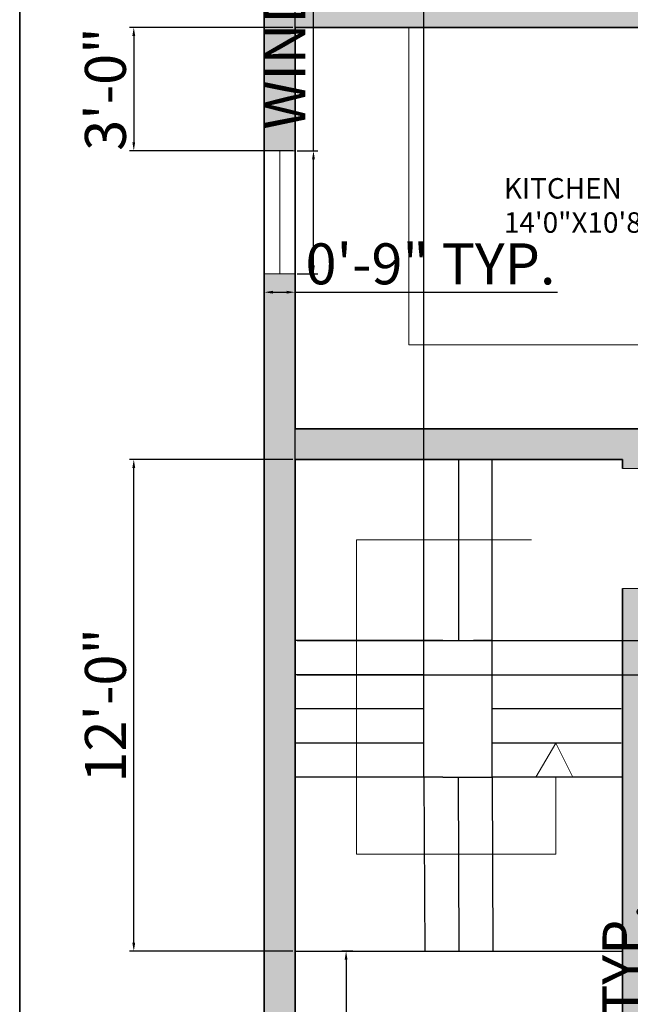
# Model space of a CAD drawing. Units: inches. Extents: x 995 to 1625, y 1005 to 1825.
# Tile 2 of 5: x 995 to 1174, y 1232 to 1521. Entities that reach past the tile are written whole.
import ezdxf

# ---------------------------------------------------------------- set-up
doc = ezdxf.new("R2010")
doc.units = ezdxf.units.IN
for name, color, linetype, lineweight in [('A-ANNO-DIMS', 2, 'Continuous', 18), ('A-ANNO-SYMB', 7, 'Continuous', 18), ('A-ANNO-TTLB', 7, 'Continuous', 35), ('A-AREA-IDEN', 7, 'Continuous', 18), ('A-DOOR', 4, 'Continuous', 18), ('A-FLOR-CASE', 8, 'Continuous', 18), ('A-FLOR-STRS', 7, 'Continuous', 25), ('A-GLAZ', 3, 'Continuous', 18), ('A-WALL', 7, 'Continuous', 35)]:
    doc.layers.add(name, color=color, linetype=linetype, lineweight=lineweight)
doc.layers.add('A-WALL-PATT', color=251, linetype='Continuous', lineweight=13, true_color=0x636466)
doc.styles.get("Standard").update_dxf_attribs({"font": 'arial.ttf'})
doc.dimstyles.new('ISO-25', dxfattribs={"dimtxt": 12, "dimasz": 2.5, "dimexe": 1.25, "dimexo": 0.625, "dimtad": 1, "dimdec": 0, "dimlunit": 3, "dimtxsty": 'Standard', "dimcen": 2.5, "dimadec": 0, "dimazin": 0, "dimtfac": 1, "dimtdec": 0, "dimtmove": 0, "dimatfit": 3, "dimfxl": 1, "dimarcsym": 0})

# ---------------------------------------------------------------- blocks, each defined once
blk = doc.blocks.new('*D1')
at = {"layer": 'A-ANNO-DIMS', "color": 0, "lineweight": -2, "transparency": 16777216}
for p, q in [((1092.78, 1247.93), (1089.58, 1247.93)), ((1090.83, 1245.43), (1090.83, 1109.93)), ((1092.78, 1107.43), (1089.58, 1107.43))]:
    blk.add_line(p, q, dxfattribs=at)
at = {"layer": 'A-ANNO-DIMS', "color": 0, "transparency": 16777216}
for points in [[(1090.41, 1245.43), (1091.25, 1245.43), (1090.83, 1247.93)], [(1090.41, 1109.93), (1091.25, 1109.93), (1090.83, 1107.43)]]:
    blk.add_solid(points, dxfattribs=at)
at = {"layer": 'Defpoints', "color": 0, "transparency": 16777216}
for p in [(1093.41, 1247.93), (1090.83, 1107.43), (1093.41, 1107.43)]:
    blk.add_point(p, dxfattribs=at)
at = {"layer": 'A-ANNO-DIMS', "color": 0, "transparency": 16777216, "insert": (1084.08, 1177.68), "char_height": 12, "attachment_point": 5, "rotation": 90}
blk.add_mtext('11\'-9"', dxfattribs=at)
blk = doc.blocks.new('WIN-36IN')
for p, q in [((0, 0), (9, 0)), ((9, 0), (4.5, 0)), ((4.5, 0), (4.5, -36)), ((4.5, -36), (0, -36)), ((0, -36), (9, -36))]:
    blk.add_line(p, q)
blk = doc.blocks.new('*D13')
at = {"layer": 'A-ANNO-DIMS', "color": 0, "lineweight": -2, "transparency": 16777216}
for p, q in [((1180.25, 1185.43), (1180.25, 1262.32)), ((1183.23, 1185.43), (1179, 1185.43)), ((1180.25, 1178.93), (1180.25, 1182.93)), ((1183.23, 1176.43), (1179, 1176.43))]:
    blk.add_line(p, q, dxfattribs=at)
at = {"layer": 'A-ANNO-DIMS', "color": 0, "transparency": 16777216}
for points in [[(1179.84, 1182.93), (1180.67, 1182.93), (1180.25, 1185.43)], [(1179.84, 1178.93), (1180.67, 1178.93), (1180.25, 1176.43)]]:
    blk.add_solid(points, dxfattribs=at)
at = {"layer": 'Defpoints', "color": 0, "transparency": 16777216}
for p in [(1180.25, 1185.43), (1183.85, 1185.43), (1183.85, 1176.43)]:
    blk.add_point(p, dxfattribs=at)
at = {"layer": 'A-ANNO-DIMS', "color": 0, "transparency": 16777216, "insert": (1173.5, 1225.13), "char_height": 12, "attachment_point": 5, "rotation": 90}
blk.add_mtext('0\'-9" TYP.', dxfattribs=at)
blk = doc.blocks.new('*D14')
at = {"layer": 'A-ANNO-DIMS', "color": 0, "lineweight": -2, "transparency": 16777216}
for p, q in [((1081.27, 1482.29), (1081.27, 1637.89)), ((1076.49, 1482.29), (1082.52, 1482.29)), ((1081.27, 1448.79), (1081.27, 1479.79)), ((1076.49, 1446.29), (1082.52, 1446.29))]:
    blk.add_line(p, q, dxfattribs=at)
at = {"layer": 'A-ANNO-DIMS', "color": 0, "transparency": 16777216}
for points in [[(1080.85, 1479.79), (1081.68, 1479.79), (1081.27, 1482.29)], [(1080.85, 1448.79), (1081.68, 1448.79), (1081.27, 1446.29)]]:
    blk.add_solid(points, dxfattribs=at)
at = {"layer": 'Defpoints', "color": 0, "transparency": 16777216}
for p in [(1075.87, 1482.29), (1081.27, 1482.29), (1075.87, 1446.29)]:
    blk.add_point(p, dxfattribs=at)
at = {"layer": 'A-ANNO-DIMS', "color": 0, "transparency": 16777216, "insert": (1074.43, 1561.34), "char_height": 12, "attachment_point": 5, "rotation": 90}
blk.add_mtext('WINDOW 3\'-0" TYP.', dxfattribs=at)
blk = doc.blocks.new('*D15')
at = {"layer": 'A-ANNO-DIMS', "color": 0, "lineweight": -2, "transparency": 16777216}
for p, q in [((1066.87, 1445.67), (1066.87, 1439.64)), ((1075.87, 1445.67), (1075.87, 1439.64)), ((1069.37, 1440.89), (1073.37, 1440.89)), ((1075.87, 1440.89), (1152.76, 1440.89))]:
    blk.add_line(p, q, dxfattribs=at)
at = {"layer": 'A-ANNO-DIMS', "color": 0, "transparency": 16777216}
for points in [[(1069.37, 1441.31), (1069.37, 1440.48), (1066.87, 1440.89)], [(1073.37, 1441.31), (1073.37, 1440.48), (1075.87, 1440.89)]]:
    blk.add_solid(points, dxfattribs=at)
at = {"layer": 'Defpoints', "color": 0, "transparency": 16777216}
for p in [(1066.87, 1446.29), (1075.87, 1446.29), (1075.87, 1440.89)]:
    blk.add_point(p, dxfattribs=at)
at = {"layer": 'A-ANNO-DIMS', "color": 0, "transparency": 16777216, "insert": (1115.56, 1447.64), "char_height": 12, "attachment_point": 5}
blk.add_mtext('0\'-9" TYP.', dxfattribs=at)
blk = doc.blocks.new('*D24')
at = {"layer": 'A-ANNO-DIMS', "color": 0, "lineweight": -2, "transparency": 16777216}
for p, q in [((1075.87, 1247.3), (1075.87, 1015.27)), ((1171.87, 1247.3), (1171.87, 1015.27)), ((1078.37, 1016.52), (1169.37, 1016.52))]:
    blk.add_line(p, q, dxfattribs=at)
at = {"layer": 'A-ANNO-DIMS', "color": 0, "transparency": 16777216}
for points in [[(1078.37, 1016.93), (1078.37, 1016.1), (1075.87, 1016.52)], [(1169.37, 1016.93), (1169.37, 1016.1), (1171.87, 1016.52)]]:
    blk.add_solid(points, dxfattribs=at)
at = {"layer": 'Defpoints', "color": 0, "transparency": 16777216}
for p in [(1075.87, 1247.93), (1171.87, 1247.93), (1171.87, 1016.52)]:
    blk.add_point(p, dxfattribs=at)
at = {"layer": 'A-ANNO-DIMS', "color": 0, "transparency": 16777216, "insert": (1123.87, 1023.27), "char_height": 12, "attachment_point": 5}
blk.add_mtext('8\'-0"', dxfattribs=at)
blk = doc.blocks.new('*D25')
at = {"layer": 'A-ANNO-DIMS', "color": 0, "lineweight": -2, "transparency": 16777216}
for p, q in [((1075.24, 1391.93), (1027.37, 1391.93)), ((1028.62, 1250.43), (1028.62, 1389.43)), ((1075.24, 1247.93), (1027.37, 1247.93))]:
    blk.add_line(p, q, dxfattribs=at)
at = {"layer": 'A-ANNO-DIMS', "color": 0, "transparency": 16777216}
for points in [[(1028.2, 1389.43), (1029.03, 1389.43), (1028.62, 1391.93)], [(1028.2, 1250.43), (1029.03, 1250.43), (1028.62, 1247.93)]]:
    blk.add_solid(points, dxfattribs=at)
at = {"layer": 'Defpoints', "color": 0, "transparency": 16777216}
for p in [(1028.62, 1391.93), (1075.87, 1391.93), (1075.87, 1247.93)]:
    blk.add_point(p, dxfattribs=at)
at = {"layer": 'A-ANNO-DIMS', "color": 0, "transparency": 16777216, "insert": (1021.86, 1319.93), "char_height": 12, "attachment_point": 5, "rotation": 90}
blk.add_mtext('12\'-0"', dxfattribs=at)
blk = doc.blocks.new('*D26')
at = {"layer": 'A-ANNO-DIMS', "color": 0, "lineweight": -2, "transparency": 16777216}
for p, q in [((1076.49, 1338.88), (1486.37, 1338.88)), ((1485.12, 1336.38), (1485.12, 1331.38)), ((1076.49, 1328.88), (1486.37, 1328.88)), ((1485.12, 1328.88), (1485.12, 1283.91))]:
    blk.add_line(p, q, dxfattribs=at)
at = {"layer": 'A-ANNO-DIMS', "color": 0, "transparency": 16777216}
for points in [[(1484.7, 1336.38), (1485.53, 1336.38), (1485.12, 1338.88)], [(1484.7, 1331.38), (1485.53, 1331.38), (1485.12, 1328.88)]]:
    blk.add_solid(points, dxfattribs=at)
at = {"layer": 'Defpoints', "color": 0, "transparency": 16777216}
for p in [(1075.87, 1338.88), (1075.87, 1328.88), (1485.12, 1328.88)]:
    blk.add_point(p, dxfattribs=at)
at = {"layer": 'A-ANNO-DIMS', "color": 0, "transparency": 16777216, "insert": (1478.36, 1305.15), "char_height": 12, "attachment_point": 5, "rotation": 90}
blk.add_mtext('0\'-10"', dxfattribs=at)
blk = doc.blocks.new('*D27')
at = {"layer": 'A-ANNO-DIMS', "color": 0, "lineweight": -2, "transparency": 16777216}
for p, q in [((1075.87, 1339.51), (1075.87, 1776.93)), ((1113.64, 1339.51), (1113.64, 1776.93)), ((1078.37, 1775.68), (1111.14, 1775.68))]:
    blk.add_line(p, q, dxfattribs=at)
at = {"layer": 'A-ANNO-DIMS', "color": 0, "transparency": 16777216}
for points in [[(1078.37, 1776.09), (1078.37, 1775.26), (1075.87, 1775.68)], [(1111.14, 1776.09), (1111.14, 1775.26), (1113.64, 1775.68)]]:
    blk.add_solid(points, dxfattribs=at)
at = {"layer": 'Defpoints', "color": 0, "transparency": 16777216}
for p in [(1113.64, 1775.68), (1075.87, 1338.88), (1113.64, 1338.88)]:
    blk.add_point(p, dxfattribs=at)
at = {"layer": 'A-ANNO-DIMS', "color": 0, "transparency": 16777216, "insert": (1094.75, 1782.43), "char_height": 12, "attachment_point": 5}
blk.add_mtext('3\'-2"', dxfattribs=at)
blk = doc.blocks.new('*D38')
at = {"layer": 'A-ANNO-DIMS', "color": 0, "lineweight": -2, "transparency": 16777216}
for p, q in [((1075.24, 1518.43), (1027.37, 1518.43)), ((1028.62, 1515.93), (1028.62, 1484.79)), ((1075.24, 1482.29), (1027.37, 1482.29))]:
    blk.add_line(p, q, dxfattribs=at)
at = {"layer": 'A-ANNO-DIMS', "color": 0, "transparency": 16777216}
for points in [[(1028.2, 1515.93), (1029.03, 1515.93), (1028.62, 1518.43)], [(1028.2, 1484.79), (1029.03, 1484.79), (1028.62, 1482.29)]]:
    blk.add_solid(points, dxfattribs=at)
at = {"layer": 'Defpoints', "color": 0, "transparency": 16777216}
for p in [(1075.87, 1518.43), (1028.62, 1482.29), (1075.87, 1482.29)]:
    blk.add_point(p, dxfattribs=at)
at = {"layer": 'A-ANNO-DIMS', "color": 0, "transparency": 16777216, "insert": (1021.86, 1500.36), "char_height": 12, "attachment_point": 5, "rotation": 90}
blk.add_mtext('3\'-0"', dxfattribs=at)

msp = doc.modelspace()

# ---------------------------------------------------------------- hatches: boundary and pattern name
at = {"layer": 'A-WALL-PATT'}
h = msp.add_hatch(color=256, dxfattribs=at)
h.dxf.hatch_style = 1
h.paths.add_polyline_path([(1446.87, 1737.43), (1066.87, 1737.43), (1066.87, 1718.28), (1075.87, 1718.28), (1075.87, 1728.43), (1171.87, 1728.43), (1171.87, 1668.43), (1165.05, 1668.43), (1165.05, 1659.43), (1219.13, 1659.43), (1219.13, 1663.93), (1219.13, 1668.43), (1180.87, 1668.43), (1180.87, 1691.88), (1180.87, 1728.43), (1249.87, 1728.43), (1258.87, 1728.43), (1332.87, 1728.43), (1332.87, 1668.43), (1311.16, 1668.43), (1311.16, 1659.43), (1346.35, 1659.43), (1346.35, 1663.93), (1346.35, 1668.43), (1341.87, 1668.43), (1341.87, 1728.43), (1437.87, 1728.43), (1437.87, 1715.56), (1446.87, 1715.56)])
h.paths.add_polyline_path([(1135.58, 1663.93), (1135.58, 1668.43), (1075.87, 1668.43), (1075.87, 1694.28), (1066.87, 1694.28), (1066.87, 1619.54), (1075.87, 1619.54), (1075.87, 1659.43), (1135.58, 1659.43)])
h.paths.add_polyline_path([(1258.87, 1659.43), (1275.16, 1659.43), (1275.16, 1663.93), (1275.16, 1668.43), (1258.87, 1668.43), (1249.87, 1668.43), (1243.74, 1668.43), (1243.74, 1659.43), (1249.87, 1659.43), (1249.87, 1527.43), (1247.75, 1527.43), (1247.75, 1518.43), (1261.81, 1518.43), (1261.81, 1527.43), (1258.87, 1527.43)])
h.paths.add_polyline_path([(1446.87, 1691.56), (1437.87, 1691.56), (1437.87, 1668.43), (1372.6, 1668.43), (1372.6, 1659.43), (1437.87, 1659.43), (1437.87, 1627.58), (1446.87, 1627.58)])
h.paths.add_polyline_path([(1446.87, 1567.58), (1437.87, 1567.58), (1437.87, 1527.43), (1291.03, 1527.43), (1291.03, 1518.43), (1380.87, 1518.43), (1380.87, 1508.92), (1389.87, 1508.92), (1389.87, 1518.43), (1437.87, 1518.43), (1437.87, 1501.62), (1446.87, 1501.62)])
h.paths.add_polyline_path([(1446.87, 1477.62), (1437.87, 1477.62), (1437.87, 1429.75), (1446.87, 1429.75)])
h.paths.add_polyline_path([(1389.87, 1441.43), (1437.87, 1441.43), (1437.87, 1450.43), (1389.87, 1450.43), (1389.87, 1481.88), (1385.37, 1481.88), (1380.87, 1481.88), (1380.87, 1385.88), (1389.87, 1385.88)])
h.paths.add_polyline_path([(1446.87, 1405.75), (1437.87, 1405.75), (1437.87, 1350.43), (1427.33, 1350.43), (1389.87, 1350.43), (1389.87, 1359.9), (1380.87, 1359.9), (1380.87, 1350.43), (1324.85, 1350.43), (1324.85, 1341.43), (1437.87, 1341.43), (1437.87, 1303.84), (1446.87, 1303.84)])
h.paths.add_polyline_path([(1311.82, 1209.43), (1281.87, 1209.43), (1281.87, 1341.43), (1291.29, 1341.43), (1291.29, 1345.93), (1291.29, 1350.43), (1244.83, 1350.43), (1244.83, 1341.43), (1272.87, 1341.43), (1272.87, 1185.43), (1268.73, 1185.43), (1268.73, 1176.43), (1272.87, 1176.43), (1281.87, 1176.43), (1281.87, 1200.43), (1311.82, 1200.43), (1311.82, 1204.93)])
h.paths.add_polyline_path([(1446.87, 1243.84), (1437.87, 1243.84), (1437.87, 1209.43), (1371.82, 1209.43), (1371.82, 1200.43), (1437.87, 1200.43), (1437.87, 1107.43), (1446.87, 1107.43)])
h.paths.add_polyline_path([(1212.11, 1185.43), (1207.85, 1185.43), (1207.85, 1176.43), (1212.11, 1176.43)], flags=17)
h.paths.add_polyline_path([(1244.73, 1185.43), (1240.24, 1185.43), (1240.24, 1176.43), (1244.73, 1176.43), (1244.73, 1180.93)])
h.paths.add_polyline_path([(1183.85, 1180.93), (1183.85, 1185.43), (1180.87, 1185.43), (1180.87, 1191.84), (1171.87, 1191.84), (1171.87, 1176.43), (1180.87, 1176.43), (1183.85, 1176.43)], flags=17)
h.paths.add_polyline_path([(1180.87, 1341.43), (1198.57, 1341.43), (1198.57, 1350.43), (1180.87, 1350.43), (1180.87, 1354.13), (1176.37, 1354.13), (1171.87, 1354.13), (1171.87, 1341.43), (1171.87, 1219.68), (1180.87, 1219.68)], flags=17)
h.paths.add_polyline_path([(1075.87, 1391.93), (1171.87, 1391.93), (1171.87, 1389.24), (1180.87, 1389.24), (1180.87, 1391.93), (1212.87, 1391.93), (1212.87, 1431.83), (1203.87, 1431.83), (1203.87, 1400.93), (1075.87, 1400.93), (1075.87, 1446.29), (1066.87, 1446.29), (1066.87, 1107.43), (1075.87, 1107.43)])
h.paths.add_polyline_path([(1218.33, 1527.43), (1075.87, 1527.43), (1075.87, 1559.54), (1066.87, 1559.54), (1066.87, 1482.29), (1075.87, 1482.29), (1075.87, 1518.43), (1203.87, 1518.43), (1203.87, 1493.65), (1212.87, 1493.65), (1212.87, 1518.43), (1218.33, 1518.43), (1218.33, 1522.93)])
h.paths.add_polyline_path([(1297.68, 1457.37), (1297.68, 1425.03), (1310.04, 1425.03), (1310.04, 1457.37)], flags=9)
h.paths.add_polyline_path([(1154.86, 1054.62), (1346.22, 1054.62), (1346.22, 1079.35), (1154.86, 1079.35)], flags=9)
h.paths.add_polyline_path([(1237.85, 1265.85), (1262.06, 1265.85), (1262.06, 1288.24), (1237.85, 1288.24)], flags=9)
h.paths.add_polyline_path([(1331.39, 1305.41), (1378, 1305.41), (1378, 1327.8), (1331.39, 1327.8)], flags=25)
h.paths.add_polyline_path([(1395.38, 1378.18), (1431.86, 1378.18), (1431.86, 1400.57), (1395.38, 1400.57)], flags=25)
h.paths.add_polyline_path([(1406.34, 1460.18), (1434.48, 1460.18), (1434.48, 1472.55), (1406.34, 1472.55)], flags=25)
h.paths.add_polyline_path([(1134.66, 1454.9), (1180.38, 1454.9), (1180.38, 1477.29), (1134.66, 1477.29)], flags=9)
h.paths.add_polyline_path([(1109.63, 1626.32), (1156.23, 1626.32), (1156.23, 1648.71), (1109.63, 1648.71)], flags=9)
h.paths.add_polyline_path([(1275.64, 1623.22), (1322.25, 1623.22), (1322.25, 1645.61), (1275.64, 1645.61)], flags=9)
h.paths.add_polyline_path([(1347.7, 1693.6), (1384.09, 1693.6), (1384.09, 1715.99), (1347.7, 1715.99)], flags=25)
h.paths.add_polyline_path([(1254.21, 1701.46), (1308.94, 1701.46), (1308.94, 1723.85), (1254.21, 1723.85)], flags=25)
h.paths.add_polyline_path([(1107.35, 1692.25), (1143.74, 1692.25), (1143.74, 1714.64), (1107.35, 1714.64)], flags=25)

# ---------------------------------------------------------------- linework, layer by layer
at = {"layer": 'A-ANNO-SYMB'}
for p, q in [((1145.19, 1368.42), (1093.88, 1368.42)), ((1093.88, 1368.42), (1093.88, 1276.35)), ((1152.25, 1308.88), (1146.44, 1298.88)), ((1157.31, 1298.88), (1152.25, 1308.88)), ((1146.44, 1298.88), (1157.31, 1298.88)), ((1152.25, 1276.35), (1152.25, 1298.88)), ((1093.88, 1276.35), (1152.25, 1276.35))]:
    msp.add_line(p, q, dxfattribs=at)
at = {"layer": 'A-ANNO-TTLB'}
msp.add_lwpolyline([(995.18, 1825.14), (1553.05, 1825.14), (1553.05, 1020.2), (995.18, 1020.2)], close=True, dxfattribs=at)
at = {"layer": 'A-DOOR'}
for p, q in [((1171.87, 1389.24), (1180.87, 1389.24)), ((1171.87, 1354.13), (1180.87, 1354.13))]:
    msp.add_line(p, q, dxfattribs=at)
at = {"layer": 'A-FLOR-CASE'}
for p, q in [((1109.19, 1518.43), (1109.19, 1425.49)), ((1109.19, 1425.49), (1203.87, 1425.49))]:
    msp.add_line(p, q, dxfattribs=at)
at = {"layer": 'A-FLOR-STRS'}
for p, q in [((1075.87, 1391.93), (1075.87, 1271.93)), ((1113.64, 1338.88), (1113.64, 1391.93)), ((1123.87, 1338.88), (1123.87, 1391.93)), ((1133.64, 1338.88), (1133.64, 1391.93)), ((1119.14, 1338.88), (1075.87, 1338.88)), ((1113.64, 1298.88), (1113.64, 1338.88)), ((1113.64, 1338.88), (1119.14, 1338.88)), ((1133.64, 1338.88), (1128.14, 1338.88)), ((1133.64, 1298.93), (1133.64, 1338.88)), ((1113.64, 1328.88), (1075.87, 1328.88)), ((1113.64, 1318.88), (1075.87, 1318.88)), ((1171.42, 1318.88), (1133.64, 1318.88)), ((1113.64, 1308.88), (1075.87, 1308.88)), ((1171.42, 1308.88), (1133.64, 1308.88)), ((1119.14, 1298.88), (1075.87, 1298.88)), ((1119.14, 1298.88), (1113.64, 1298.88)), ((1113.64, 1298.84), (1113.87, 1247.88)), ((1119.14, 1298.88), (1128.14, 1298.88)), ((1123.64, 1298.88), (1123.87, 1247.93)), ((1128.14, 1298.88), (1133.64, 1298.93)), ((1133.64, 1298.93), (1133.87, 1247.97)), ((1171.87, 1298.88), (1133.64, 1298.88)), ((1075.87, 1271.93), (1075.87, 1247.93)), ((1075.87, 1247.93), (1171.87, 1247.93))]:
    msp.add_line(p, q, dxfattribs=at)
msp.add_lwpolyline([(1119.14, 1338.88), (1128.14, 1338.88)], dxfattribs=at)
at = {"layer": 'A-WALL'}
for p, q in [((1066.87, 1737.43), (1066.87, 1107.43)), ((1066.87, 1737.43), (1066.87, 1107.43)), ((1066.87, 1737.43), (1066.87, 1107.43)), ((1075.87, 1518.43), (1203.87, 1518.43)), ((1075.87, 1518.43), (1075.87, 1400.93)), ((1066.87, 1400.93), (1066.87, 1391.93)), ((1203.87, 1400.93), (1075.87, 1400.93)), ((1075.87, 1391.93), (1171.87, 1391.93)), ((1075.87, 1391.93), (1075.87, 1107.43)), ((1171.87, 1389.24), (1171.87, 1391.93)), ((1171.87, 1341.43), (1171.87, 1354.13)), ((1171.87, 1341.43), (1171.87, 1219.68))]:
    msp.add_line(p, q, dxfattribs=at)

# ---------------------------------------------------------------- block references
at = {"layer": 'A-GLAZ'}
msp.add_blockref('WIN-36IN', (1066.87, 1482.29), dxfattribs=at)

# ---------------------------------------------------------------- texts
at = {"layer": 'A-AREA-IDEN', "insert": (1137.08, 1474.3), "char_height": 6, "attachment_point": 1}
msp.add_mtext_dynamic_manual_height_columns('KITCHEN\\P14\'0"X10\'8"', width=168.4596, gutter_width=12.5, heights=[0], dxfattribs=at)

# ---------------------------------------------------------------- dimensions: what is measured, and where the dimension line sits
at = {"layer": 'A-ANNO-DIMS'}
for base, p1, p2, picture, middle in [((1113.64, 1775.68), (1075.87, 1338.88), (1113.64, 1338.88), '*D27', (1094.75, 1782.43)), ((1171.87, 1016.52), (1075.87, 1247.93), (1171.87, 1247.93), '*D24', (1123.87, 1023.27))]:
    dim = msp.add_linear_dim(base=base, p1=p1, p2=p2, dimstyle='ISO-25', override={"dimdec": 1, "dimlfac": 1, "dimrnd": 0, "dimzin": 1, "dimdsep": 46, "dimlunit": 4, "dimfrac": 2}, dxfattribs=at)
    dim.commit()
    dim.dimension.update_dxf_attribs({"geometry": picture, "text_midpoint": middle})
for base, p1, p2, text, picture, middle in [((1081.27, 1482.29), (1075.87, 1446.29), (1075.87, 1482.29), 'WINDOW <> TYP.', '*D14', (1074.43, 1561.34)), ((1180.25, 1185.43), (1183.85, 1176.43), (1183.85, 1185.43), '<> TYP.', '*D13', (1173.5, 1225.13))]:
    dim = msp.add_linear_dim(base=base, p1=p1, p2=p2, angle=90, text=text, dimstyle='ISO-25', override={"dimdec": 1, "dimlfac": 1, "dimrnd": 0, "dimzin": 1, "dimdsep": 46, "dimlunit": 4, "dimfrac": 2}, dxfattribs=at)
    dim.commit()
    dim.dimension.update_dxf_attribs({"geometry": picture, "text_midpoint": middle})
for base, p1, p2, picture, middle in [((1028.62, 1482.29), (1075.87, 1518.43), (1075.87, 1482.29), '*D38', (1021.86, 1500.36)), ((1028.62, 1391.93), (1075.87, 1247.93), (1075.87, 1391.93), '*D25', (1021.86, 1319.93)), ((1485.12, 1328.88), (1075.87, 1338.88), (1075.87, 1328.88), '*D26', (1478.36, 1305.15))]:
    dim = msp.add_linear_dim(base=base, p1=p1, p2=p2, angle=90, dimstyle='ISO-25', override={"dimdec": 1, "dimlfac": 1, "dimrnd": 0, "dimzin": 1, "dimdsep": 46, "dimlunit": 4, "dimfrac": 2}, dxfattribs=at)
    dim.commit()
    dim.dimension.update_dxf_attribs({"geometry": picture, "text_midpoint": middle})
dim = msp.add_linear_dim(base=(1075.87, 1440.89), p1=(1066.87, 1446.29), p2=(1075.87, 1446.29), text='<> TYP.', dimstyle='ISO-25', override={"dimdec": 1, "dimlfac": 1, "dimrnd": 0, "dimzin": 1, "dimdsep": 46, "dimlunit": 4, "dimfrac": 2}, dxfattribs=at)
dim.commit()
dim.dimension.update_dxf_attribs({"geometry": '*D15', "text_midpoint": (1115.56, 1447.64)})
dim = msp.add_linear_dim(base=(1090.8307, 1107.4271), p1=(1093.4057, 1247.928), p2=(1093.4057, 1107.4271), angle=90, dimstyle='ISO-25', override={"dimclrd": 0, "dimclre": 0, "dimclrt": 0}, dxfattribs=at)
dim.commit()
dim.dimension.update_dxf_attribs({"geometry": '*D1', "text_midpoint": (1090.8307, 1177.6775), "dimtype": 160})

doc.saveas('drawing.dxf')
